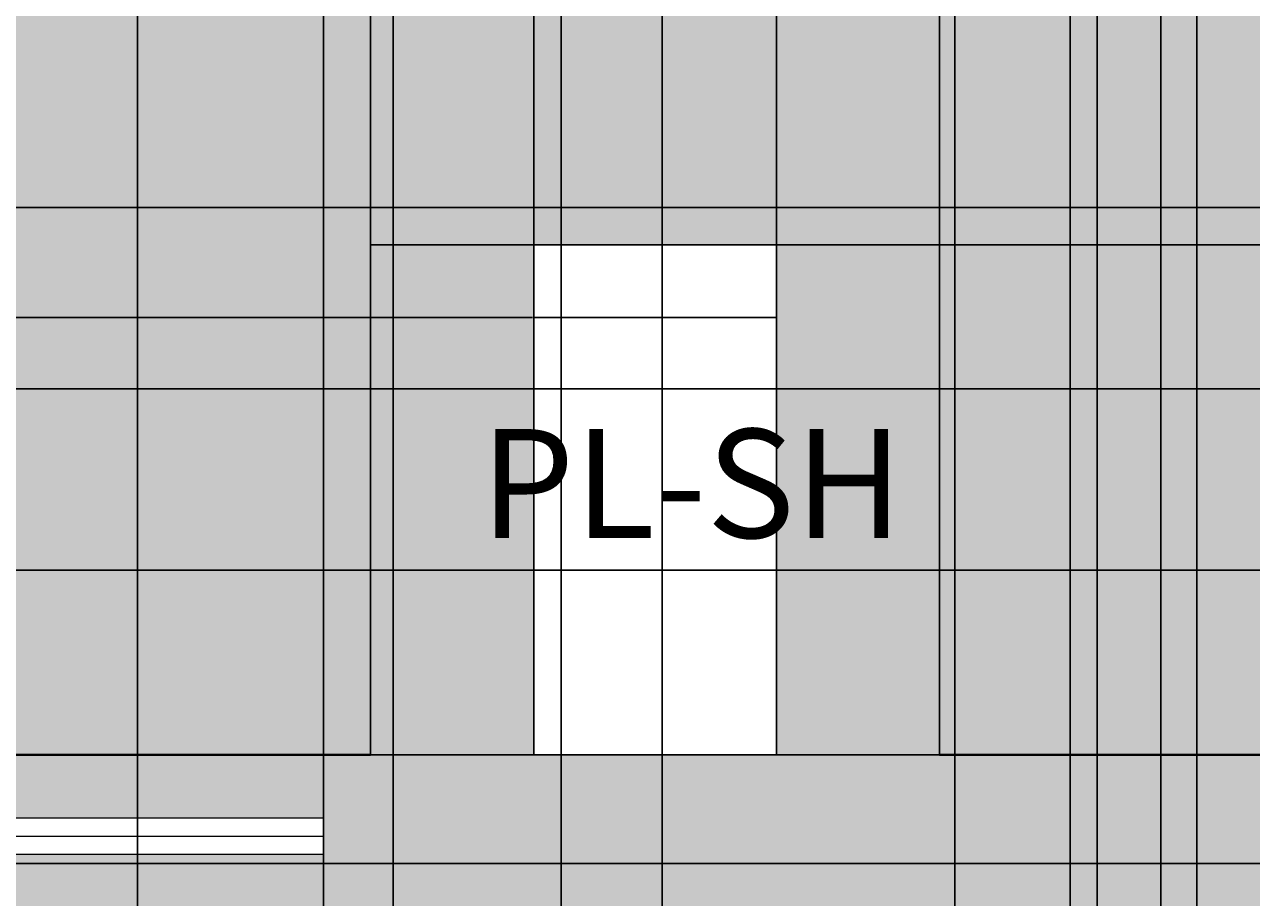
# Model space of a CAD drawing. Units: inches. Extents: x 818 to 1898, y 976 to 2364.
# Tile 77 of 96: x 1372 to 1439, y 2045 to 2093. Entities that reach past the tile are written whole.
import ezdxf

# ---------------------------------------------------------------- set-up
doc = ezdxf.new("R2010")
doc.units = ezdxf.units.IN
doc.header["$LTSCALE"] = 5
doc.header["$MEASUREMENT"] = 0
for name, color, linetype, lineweight in [('A-ANNO-DIMS', 2, 'Continuous', 18), ('A-ANNO-TEXT', 7, 'Continuous', 18), ('A-FLOR-SHFT', 7, 'Continuous', 25), ('A-GLAZ', 4, 'Continuous', 18), ('A-WALL', 7, 'Continuous', 40)]:
    doc.layers.add(name, color=color, linetype=linetype, lineweight=lineweight)
for name, color, linetype, lineweight, true_color in [('A-GLAZ-PATT', 141, 'Continuous', 9, 0xadddf7), ('A-WALL-PATT', 251, 'Continuous', 13, 0x636466), ('L-PLNT-PATT', 114, 'Continuous', 9, 0x139b48)]:
    doc.layers.add(name, color=color, linetype=linetype, lineweight=lineweight, true_color=true_color)
doc.styles.get("Standard").update_dxf_attribs({"font": 'arial.ttf'})
doc.dimstyles.get("Standard").update_dxf_attribs({"dimtxt": 0.18, "dimasz": 0.18, "dimexe": 0.18, "dimexo": 0.0625, "dimgap": 0.09, "dimtad": 0, "dimtih": 1, "dimtoh": 1, "dimdec": 4, "dimzin": 0, "dimdsep": 46, "dimtxsty": 'Standard', "dimcen": 0.09, "dimadec": 0, "dimazin": 0, "dimtfac": 1, "dimtdec": 4, "dimtofl": 0, "dimtmove": 0, "dimatfit": 3, "dimfxl": 1, "dimtolj": 1, "dimtzin": 0, "dimarcsym": 0})

# ---------------------------------------------------------------- blocks, each defined once
blk = doc.blocks.new('*D61')
at = {"layer": 'A-ANNO-DIMS', "color": 0, "lineweight": -2, "ltscale": 5, "transparency": 16777216}
for p, q in [((1071.725, 1203.027), (1071.725, 2363.873)), ((1071.905, 2363.693), (1250.936, 2363.693)), ((1430.545, 2363.693), (1251.514, 2363.693)), ((1430.725, 1203.027), (1430.725, 2363.873))]:
    blk.add_line(p, q, dxfattribs=at)
at = {"layer": 'A-ANNO-DIMS', "color": 0, "ltscale": 5, "transparency": 16777216}
for points in [[(1071.905, 2363.723), (1071.905, 2363.663), (1071.725, 2363.693)], [(1430.545, 2363.723), (1430.545, 2363.663), (1430.725, 2363.693)]]:
    blk.add_solid(points, dxfattribs=at)
at = {"layer": 'Defpoints', "color": 0, "ltscale": 5, "transparency": 16777216}
for p in [(1430.725, 2363.693), (1071.725, 1202.964), (1430.725, 1202.964)]:
    blk.add_point(p, dxfattribs=at)
at = {"layer": 'A-ANNO-DIMS', "color": 0, "ltscale": 5, "transparency": 16777216, "insert": (1251.225, 2363.693), "char_height": 0.18, "attachment_point": 5}
blk.add_mtext('\\A1;359', dxfattribs=at)
blk = doc.blocks.new('*D64')
at = {"layer": 'A-ANNO-DIMS', "color": 0, "lineweight": -2, "ltscale": 5, "transparency": 16777216}
for p, q in [((1197.725, 1501.141), (1197.725, 2363.873)), ((1197.905, 2363.693), (1313.935, 2363.693)), ((1430.545, 2363.693), (1314.516, 2363.693)), ((1430.725, 1501.141), (1430.725, 2363.873))]:
    blk.add_line(p, q, dxfattribs=at)
at = {"layer": 'A-ANNO-DIMS', "color": 0, "ltscale": 5, "transparency": 16777216}
for points in [[(1197.905, 2363.723), (1197.905, 2363.663), (1197.725, 2363.693)], [(1430.545, 2363.723), (1430.545, 2363.663), (1430.725, 2363.693)]]:
    blk.add_solid(points, dxfattribs=at)
at = {"layer": 'Defpoints', "color": 0, "ltscale": 5, "transparency": 16777216}
for p in [(1430.725, 2363.693), (1197.725, 1501.078), (1430.725, 1501.078)]:
    blk.add_point(p, dxfattribs=at)
at = {"layer": 'A-ANNO-DIMS', "color": 0, "ltscale": 5, "transparency": 16777216, "insert": (1314.225, 2363.693), "char_height": 0.18, "attachment_point": 5}
blk.add_mtext('\\A1;233', dxfattribs=at)
blk = doc.blocks.new('*D85')
at = {"layer": 'A-ANNO-DIMS', "color": 0, "lineweight": -2, "ltscale": 5, "transparency": 16777216}
for p, q in [((1258.788, 2053.078), (1897.916, 2053.078)), ((1897.736, 2052.898), (1897.736, 1876.76)), ((1897.736, 1700.258), (1897.736, 1876.396)), ((1258.788, 1700.078), (1897.916, 1700.078))]:
    blk.add_line(p, q, dxfattribs=at)
at = {"layer": 'A-ANNO-DIMS', "color": 0, "ltscale": 5, "transparency": 16777216}
for points in [[(1897.706, 2052.898), (1897.766, 2052.898), (1897.736, 2053.078)], [(1897.706, 1700.258), (1897.766, 1700.258), (1897.736, 1700.078)]]:
    blk.add_solid(points, dxfattribs=at)
at = {"layer": 'Defpoints', "color": 0, "ltscale": 5, "transparency": 16777216}
for p in [(1258.725, 2053.078), (1897.736, 2053.078), (1258.725, 1700.078)]:
    blk.add_point(p, dxfattribs=at)
at = {"layer": 'A-ANNO-DIMS', "color": 0, "ltscale": 5, "transparency": 16777216, "insert": (1897.736, 1876.578), "char_height": 0.18, "attachment_point": 5}
blk.add_mtext('\\A1;353', dxfattribs=at)
blk = doc.blocks.new('*D86')
at = {"layer": 'A-ANNO-DIMS', "color": 0, "lineweight": -2, "ltscale": 5, "transparency": 16777216}
for p, q in [((1258.725, 2053.141), (1258.725, 2363.873)), ((1258.905, 2363.693), (1486.433, 2363.693)), ((1714.545, 2363.693), (1487.018, 2363.693)), ((1714.725, 2053.141), (1714.725, 2363.873))]:
    blk.add_line(p, q, dxfattribs=at)
at = {"layer": 'A-ANNO-DIMS', "color": 0, "ltscale": 5, "transparency": 16777216}
for points in [[(1258.905, 2363.723), (1258.905, 2363.663), (1258.725, 2363.693)], [(1714.545, 2363.723), (1714.545, 2363.663), (1714.725, 2363.693)]]:
    blk.add_solid(points, dxfattribs=at)
at = {"layer": 'Defpoints', "color": 0, "ltscale": 5, "transparency": 16777216}
for p in [(1714.725, 2363.693), (1258.725, 2053.078), (1714.725, 2053.078)]:
    blk.add_point(p, dxfattribs=at)
at = {"layer": 'A-ANNO-DIMS', "color": 0, "ltscale": 5, "transparency": 16777216, "insert": (1486.725, 2363.693), "char_height": 0.18, "attachment_point": 5}
blk.add_mtext('\\A1;456', dxfattribs=at)
blk = doc.blocks.new('*D98')
at = {"layer": 'A-ANNO-DIMS', "color": 0, "lineweight": -2, "ltscale": 5, "transparency": 16777216}
for p, q in [((1338.541, 1071.118), (1338.541, 2363.873)), ((1338.721, 2363.693), (1364.815, 2363.693)), ((1391.696, 2363.693), (1365.602, 2363.693)), ((1391.876, 1071.118), (1391.876, 2363.873))]:
    blk.add_line(p, q, dxfattribs=at)
at = {"layer": 'A-ANNO-DIMS', "color": 0, "ltscale": 5, "transparency": 16777216}
for points in [[(1338.721, 2363.723), (1338.721, 2363.663), (1338.541, 2363.693)], [(1391.696, 2363.723), (1391.696, 2363.663), (1391.876, 2363.693)]]:
    blk.add_solid(points, dxfattribs=at)
at = {"layer": 'Defpoints', "color": 0, "ltscale": 5, "transparency": 16777216}
for p in [(1391.876, 2363.693), (1338.541, 1071.055), (1391.876, 1071.055)]:
    blk.add_point(p, dxfattribs=at)
at = {"layer": 'A-ANNO-DIMS', "color": 0, "ltscale": 5, "transparency": 16777216, "insert": (1365.208, 2363.693), "char_height": 0.18, "attachment_point": 5}
blk.add_mtext('\\A1;53.33', dxfattribs=at)
blk = doc.blocks.new('*D99')
at = {"layer": 'A-ANNO-DIMS', "color": 0, "lineweight": -2, "ltscale": 5, "transparency": 16777216}
for p, q in [((1391.876, 1071.118), (1391.876, 2363.873)), ((1392.056, 2363.693), (1420.454, 2363.693)), ((1449.64, 2363.693), (1421.241, 2363.693)), ((1449.82, 1071.118), (1449.82, 2363.873))]:
    blk.add_line(p, q, dxfattribs=at)
at = {"layer": 'A-ANNO-DIMS', "color": 0, "ltscale": 5, "transparency": 16777216}
for points in [[(1392.056, 2363.723), (1392.056, 2363.663), (1391.876, 2363.693)], [(1449.64, 2363.723), (1449.64, 2363.663), (1449.82, 2363.693)]]:
    blk.add_solid(points, dxfattribs=at)
at = {"layer": 'Defpoints', "color": 0, "ltscale": 5, "transparency": 16777216}
for p in [(1449.82, 2363.693), (1391.876, 1071.055), (1449.82, 1071.055)]:
    blk.add_point(p, dxfattribs=at)
at = {"layer": 'A-ANNO-DIMS', "color": 0, "ltscale": 5, "transparency": 16777216, "insert": (1420.848, 2363.693), "char_height": 0.18, "attachment_point": 5}
blk.add_mtext('\\A1;57.94', dxfattribs=at)
blk = doc.blocks.new('*D141')
at = {"layer": 'A-ANNO-DIMS', "color": 0, "lineweight": -2, "ltscale": 5, "transparency": 16777216}
for p, q in [((1218.174, 2083.262), (1897.916, 2083.262)), ((1897.736, 2083.082), (1897.736, 2073.444)), ((1897.736, 2063.442), (1897.736, 2073.08)), ((1198.174, 2063.262), (1897.916, 2063.262))]:
    blk.add_line(p, q, dxfattribs=at)
at = {"layer": 'A-ANNO-DIMS', "color": 0, "ltscale": 5, "transparency": 16777216}
for points in [[(1897.706, 2083.082), (1897.766, 2083.082), (1897.736, 2083.262)], [(1897.706, 2063.442), (1897.766, 2063.442), (1897.736, 2063.262)]]:
    blk.add_solid(points, dxfattribs=at)
at = {"layer": 'Defpoints', "color": 0, "ltscale": 5, "transparency": 16777216}
for p in [(1218.111, 2083.262), (1198.111, 2063.262), (1897.736, 2063.262)]:
    blk.add_point(p, dxfattribs=at)
at = {"layer": 'A-ANNO-DIMS', "color": 0, "ltscale": 5, "transparency": 16777216, "insert": (1897.736, 2073.262), "char_height": 0.18, "attachment_point": 5}
blk.add_mtext('\\A1;20', dxfattribs=at)
blk = doc.blocks.new('*D142')
at = {"layer": 'A-ANNO-DIMS', "color": 0, "lineweight": -2, "ltscale": 5, "transparency": 16777216}
for p, q in [((1208.174, 2073.262), (1897.916, 2073.262)), ((1897.736, 2073.082), (1897.736, 2068.444)), ((1897.736, 2063.442), (1897.736, 2068.08)), ((1198.174, 2063.262), (1897.916, 2063.262))]:
    blk.add_line(p, q, dxfattribs=at)
at = {"layer": 'A-ANNO-DIMS', "color": 0, "ltscale": 5, "transparency": 16777216}
for points in [[(1897.706, 2073.082), (1897.766, 2073.082), (1897.736, 2073.262)], [(1897.706, 2063.442), (1897.766, 2063.442), (1897.736, 2063.262)]]:
    blk.add_solid(points, dxfattribs=at)
at = {"layer": 'Defpoints', "color": 0, "ltscale": 5, "transparency": 16777216}
for p in [(1208.111, 2073.262), (1897.736, 2073.262), (1198.111, 2063.262)]:
    blk.add_point(p, dxfattribs=at)
at = {"layer": 'A-ANNO-DIMS', "color": 0, "ltscale": 5, "transparency": 16777216, "insert": (1897.736, 2068.262), "char_height": 0.18, "attachment_point": 5}
blk.add_mtext('\\A1;10', dxfattribs=at)
blk = doc.blocks.new('*D161')
at = {"layer": 'A-ANNO-DIMS', "color": 0, "lineweight": -2, "ltscale": 5, "transparency": 16777216}
for p, q in [((1429.225, 1876.141), (1429.225, 2363.873)), ((1429.405, 2363.693), (1509.589, 2363.693)), ((1590.545, 2363.693), (1510.361, 2363.693)), ((1590.725, 1876.141), (1590.725, 2363.873))]:
    blk.add_line(p, q, dxfattribs=at)
at = {"layer": 'A-ANNO-DIMS', "color": 0, "ltscale": 5, "transparency": 16777216}
for points in [[(1429.405, 2363.723), (1429.405, 2363.663), (1429.225, 2363.693)], [(1590.545, 2363.723), (1590.545, 2363.663), (1590.725, 2363.693)]]:
    blk.add_solid(points, dxfattribs=at)
at = {"layer": 'Defpoints', "color": 0, "ltscale": 5, "transparency": 16777216}
for p in [(1590.725, 2363.693), (1429.225, 1876.078), (1590.725, 1876.078)]:
    blk.add_point(p, dxfattribs=at)
at = {"layer": 'A-ANNO-DIMS', "color": 0, "ltscale": 5, "transparency": 16777216, "insert": (1509.975, 2363.693), "char_height": 0.18, "attachment_point": 5}
blk.add_mtext('\\A1;161.5', dxfattribs=at)
blk = doc.blocks.new('*D166')
at = {"layer": 'A-ANNO-DIMS', "color": 0, "lineweight": -2, "ltscale": 5, "transparency": 16777216}
for p, q in [((1401.146, 1510.141), (1401.146, 2363.873)), ((1401.326, 2363.693), (1415.54, 2363.693)), ((1430.545, 2363.693), (1416.331, 2363.693)), ((1430.725, 1510.141), (1430.725, 2363.873))]:
    blk.add_line(p, q, dxfattribs=at)
at = {"layer": 'A-ANNO-DIMS', "color": 0, "ltscale": 5, "transparency": 16777216}
for points in [[(1401.326, 2363.723), (1401.326, 2363.663), (1401.146, 2363.693)], [(1430.545, 2363.723), (1430.545, 2363.663), (1430.725, 2363.693)]]:
    blk.add_solid(points, dxfattribs=at)
at = {"layer": 'Defpoints', "color": 0, "ltscale": 5, "transparency": 16777216}
for p in [(1430.725, 2363.693), (1401.146, 1510.078), (1430.725, 1510.078)]:
    blk.add_point(p, dxfattribs=at)
at = {"layer": 'A-ANNO-DIMS', "color": 0, "ltscale": 5, "transparency": 16777216, "insert": (1415.936, 2363.693), "char_height": 0.18, "attachment_point": 5}
blk.add_mtext('\\A1;29.58', dxfattribs=at)
blk = doc.blocks.new('*D191')
at = {"layer": 'A-ANNO-DIMS', "color": 0, "lineweight": -2, "ltscale": 5, "transparency": 16777216}
for p, q in [((1434.225, 1409.115), (1434.225, 2363.873)), ((1434.405, 2363.693), (1435.076, 2363.693)), ((1436.045, 2363.693), (1435.375, 2363.693)), ((1436.225, 1409.115), (1436.225, 2363.873))]:
    blk.add_line(p, q, dxfattribs=at)
at = {"layer": 'A-ANNO-DIMS', "color": 0, "ltscale": 5, "transparency": 16777216}
for points in [[(1434.405, 2363.723), (1434.405, 2363.663), (1434.225, 2363.693)], [(1436.045, 2363.723), (1436.045, 2363.663), (1436.225, 2363.693)]]:
    blk.add_solid(points, dxfattribs=at)
at = {"layer": 'Defpoints', "color": 0, "ltscale": 5, "transparency": 16777216}
for p in [(1436.225, 2363.693), (1434.225, 1409.052), (1436.225, 1409.052)]:
    blk.add_point(p, dxfattribs=at)
at = {"layer": 'A-ANNO-DIMS', "color": 0, "ltscale": 5, "transparency": 16777216, "insert": (1435.225, 2363.693), "char_height": 0.18, "attachment_point": 5}
blk.add_mtext('\\A1;2', dxfattribs=at)
blk = doc.blocks.new('*D252')
at = {"layer": 'A-ANNO-DIMS', "color": 0, "lineweight": -2, "ltscale": 5, "transparency": 16777216}
for p, q in [((1330.305, 2053.016), (1330.305, 975.663)), ((1388.031, 2053.016), (1388.031, 975.663)), ((1330.485, 975.843), (1358.775, 975.843)), ((1387.851, 975.843), (1359.562, 975.843))]:
    blk.add_line(p, q, dxfattribs=at)
at = {"layer": 'A-ANNO-DIMS', "color": 0, "ltscale": 5, "transparency": 16777216}
for points in [[(1330.485, 975.873), (1330.485, 975.813), (1330.305, 975.843)], [(1387.851, 975.873), (1387.851, 975.813), (1388.031, 975.843)]]:
    blk.add_solid(points, dxfattribs=at)
at = {"layer": 'Defpoints', "color": 0, "ltscale": 5, "transparency": 16777216}
for p in [(1330.305, 2053.078), (1388.031, 2053.078), (1388.031, 975.843)]:
    blk.add_point(p, dxfattribs=at)
at = {"layer": 'A-ANNO-DIMS', "color": 0, "ltscale": 5, "transparency": 16777216, "insert": (1359.168, 975.843), "char_height": 0.18, "attachment_point": 5}
blk.add_mtext('\\A1;57.73', dxfattribs=at)
blk = doc.blocks.new('*D255')
at = {"layer": 'A-ANNO-DIMS', "color": 0, "lineweight": -2, "ltscale": 5, "transparency": 16777216}
for p, q in [((1388.031, 2053.141), (1388.031, 2363.873)), ((1388.211, 2363.693), (1388.939, 2363.693)), ((1390.456, 2363.693), (1389.728, 2363.693)), ((1390.636, 2053.141), (1390.636, 2363.873))]:
    blk.add_line(p, q, dxfattribs=at)
at = {"layer": 'A-ANNO-DIMS', "color": 0, "ltscale": 5, "transparency": 16777216}
for points in [[(1388.211, 2363.723), (1388.211, 2363.663), (1388.031, 2363.693)], [(1390.456, 2363.723), (1390.456, 2363.663), (1390.636, 2363.693)]]:
    blk.add_solid(points, dxfattribs=at)
at = {"layer": 'Defpoints', "color": 0, "ltscale": 5, "transparency": 16777216}
for p in [(1390.636, 2363.693), (1388.031, 2053.078), (1390.636, 2053.078)]:
    blk.add_point(p, dxfattribs=at)
at = {"layer": 'A-ANNO-DIMS', "color": 0, "ltscale": 5, "transparency": 16777216, "insert": (1389.334, 2363.693), "char_height": 0.18, "attachment_point": 5}
blk.add_mtext('\\A1;2.604', dxfattribs=at)
blk = doc.blocks.new('*D256')
at = {"layer": 'A-ANNO-DIMS', "color": 0, "lineweight": -2, "ltscale": 5, "transparency": 16777216}
for p, q in [((1399.636, 2053.141), (1399.636, 2363.873)), ((1399.816, 2363.693), (1405.873, 2363.693)), ((1412.84, 2363.693), (1406.783, 2363.693)), ((1413.02, 2077.251), (1413.02, 2363.873))]:
    blk.add_line(p, q, dxfattribs=at)
at = {"layer": 'A-ANNO-DIMS', "color": 0, "ltscale": 5, "transparency": 16777216}
for points in [[(1399.816, 2363.723), (1399.816, 2363.663), (1399.636, 2363.693)], [(1412.84, 2363.723), (1412.84, 2363.663), (1413.02, 2363.693)]]:
    blk.add_solid(points, dxfattribs=at)
at = {"layer": 'Defpoints', "color": 0, "ltscale": 5, "transparency": 16777216}
for p in [(1413.02, 2363.693), (1413.02, 2077.188), (1399.636, 2053.078)]:
    blk.add_point(p, dxfattribs=at)
at = {"layer": 'A-ANNO-DIMS', "color": 0, "ltscale": 5, "transparency": 16777216, "insert": (1406.328, 2363.693), "char_height": 0.18, "attachment_point": 5}
blk.add_mtext('\\A1;13.384', dxfattribs=at)
blk = doc.blocks.new('*D257')
at = {"layer": 'A-ANNO-DIMS', "color": 0, "lineweight": -2, "ltscale": 5, "transparency": 16777216}
for p, q in [((1399.573, 2077.188), (818.026, 2077.188)), ((818.206, 2077.008), (818.206, 2065.314)), ((818.206, 2053.258), (818.206, 2064.953)), ((1399.573, 2053.078), (818.026, 2053.078))]:
    blk.add_line(p, q, dxfattribs=at)
at = {"layer": 'A-ANNO-DIMS', "color": 0, "ltscale": 5, "transparency": 16777216}
for points in [[(818.176, 2077.008), (818.236, 2077.008), (818.206, 2077.188)], [(818.176, 2053.258), (818.236, 2053.258), (818.206, 2053.078)]]:
    blk.add_solid(points, dxfattribs=at)
at = {"layer": 'Defpoints', "color": 0, "ltscale": 5, "transparency": 16777216}
for p in [(818.206, 2077.188), (1399.636, 2077.188), (1399.636, 2053.078)]:
    blk.add_point(p, dxfattribs=at)
at = {"layer": 'A-ANNO-DIMS', "color": 0, "ltscale": 5, "transparency": 16777216, "insert": (818.206, 2065.133), "char_height": 0.18, "attachment_point": 5}
blk.add_mtext('\\A1;24.11', dxfattribs=at)
blk = doc.blocks.new('*D258')
at = {"layer": 'A-ANNO-DIMS', "color": 0, "lineweight": -2, "ltscale": 5, "transparency": 16777216}
for p, q in [((1422.02, 2053.141), (1422.02, 2363.873)), ((1422.2, 2363.693), (1453.264, 2363.693)), ((1484.942, 2363.693), (1453.878, 2363.693)), ((1485.122, 2053.141), (1485.122, 2363.873))]:
    blk.add_line(p, q, dxfattribs=at)
at = {"layer": 'A-ANNO-DIMS', "color": 0, "ltscale": 5, "transparency": 16777216}
for points in [[(1422.2, 2363.723), (1422.2, 2363.663), (1422.02, 2363.693)], [(1484.942, 2363.723), (1484.942, 2363.663), (1485.122, 2363.693)]]:
    blk.add_solid(points, dxfattribs=at)
at = {"layer": 'Defpoints', "color": 0, "ltscale": 5, "transparency": 16777216}
for p in [(1485.122, 2363.693), (1422.02, 2053.078), (1485.122, 2053.078)]:
    blk.add_point(p, dxfattribs=at)
at = {"layer": 'A-ANNO-DIMS', "color": 0, "ltscale": 5, "transparency": 16777216, "insert": (1453.571, 2363.693), "char_height": 0.18, "attachment_point": 5}
blk.add_mtext('\\A1;63.1', dxfattribs=at)
blk = doc.blocks.new('*D266')
at = {"layer": 'A-ANNO-DIMS', "color": 0, "lineweight": -2, "ltscale": 5, "transparency": 16777216}
for p, q in [((1780.439, 2053.078), (818.026, 2053.078)), ((818.206, 2052.898), (818.206, 2050.26)), ((818.206, 2047.258), (818.206, 2049.896)), ((1780.439, 2047.078), (818.026, 2047.078))]:
    blk.add_line(p, q, dxfattribs=at)
at = {"layer": 'A-ANNO-DIMS', "color": 0, "ltscale": 5, "transparency": 16777216}
for points in [[(818.176, 2052.898), (818.236, 2052.898), (818.206, 2053.078)], [(818.176, 2047.258), (818.236, 2047.258), (818.206, 2047.078)]]:
    blk.add_solid(points, dxfattribs=at)
at = {"layer": 'Defpoints', "color": 0, "ltscale": 5, "transparency": 16777216}
for p in [(1780.502, 2053.078), (818.206, 2047.078), (1780.502, 2047.078)]:
    blk.add_point(p, dxfattribs=at)
at = {"layer": 'A-ANNO-DIMS', "color": 0, "ltscale": 5, "transparency": 16777216, "insert": (818.206, 2050.078), "char_height": 0.18, "attachment_point": 5}
blk.add_mtext('\\A1;6', dxfattribs=at)
blk = doc.blocks.new('*D273')
at = {"layer": 'A-ANNO-DIMS', "color": 0, "lineweight": -2, "ltscale": 5, "transparency": 16777216}
for p, q in [((1406.725, 1587.479), (1406.725, 2363.873)), ((1406.905, 2363.693), (1418.505, 2363.693)), ((1430.545, 2363.693), (1418.945, 2363.693)), ((1430.725, 1587.479), (1430.725, 2363.873))]:
    blk.add_line(p, q, dxfattribs=at)
at = {"layer": 'A-ANNO-DIMS', "color": 0, "ltscale": 5, "transparency": 16777216}
for points in [[(1406.905, 2363.723), (1406.905, 2363.663), (1406.725, 2363.693)], [(1430.545, 2363.723), (1430.545, 2363.663), (1430.725, 2363.693)]]:
    blk.add_solid(points, dxfattribs=at)
at = {"layer": 'Defpoints', "color": 0, "ltscale": 5, "transparency": 16777216}
for p in [(1430.725, 2363.693), (1406.725, 1587.416), (1430.725, 1587.416)]:
    blk.add_point(p, dxfattribs=at)
at = {"layer": 'A-ANNO-DIMS', "color": 0, "ltscale": 5, "transparency": 16777216, "insert": (1418.725, 2363.693), "char_height": 0.18, "attachment_point": 5}
blk.add_mtext('\\A1;24', dxfattribs=at)
blk = doc.blocks.new('*D274')
at = {"layer": 'A-ANNO-DIMS', "color": 0, "lineweight": -2, "ltscale": 5, "transparency": 16777216}
for p, q in [((1311.025, 1897.929), (1311.025, 2363.873)), ((1311.205, 2363.693), (1344.007, 2363.693)), ((1377.599, 2363.693), (1344.797, 2363.693)), ((1377.779, 1897.929), (1377.779, 2363.873))]:
    blk.add_line(p, q, dxfattribs=at)
at = {"layer": 'A-ANNO-DIMS', "color": 0, "ltscale": 5, "transparency": 16777216}
for points in [[(1311.205, 2363.723), (1311.205, 2363.663), (1311.025, 2363.693)], [(1377.599, 2363.723), (1377.599, 2363.663), (1377.779, 2363.693)]]:
    blk.add_solid(points, dxfattribs=at)
at = {"layer": 'Defpoints', "color": 0, "ltscale": 5, "transparency": 16777216}
for p in [(1377.779, 2363.693), (1311.025, 1897.866), (1377.779, 1897.866)]:
    blk.add_point(p, dxfattribs=at)
at = {"layer": 'A-ANNO-DIMS', "color": 0, "ltscale": 5, "transparency": 16777216, "insert": (1344.402, 2363.693), "char_height": 0.18, "attachment_point": 5}
blk.add_mtext('\\A1;66.75', dxfattribs=at)
blk = doc.blocks.new('*D281')
at = {"layer": 'A-ANNO-DIMS', "color": 0, "lineweight": -2, "ltscale": 5, "transparency": 16777216}
for p, q in [((1250.303, 1913.703), (1250.303, 2363.873)), ((1250.483, 2363.693), (1420.121, 2363.693)), ((1590.545, 2363.693), (1420.907, 2363.693)), ((1590.725, 2011.141), (1590.725, 2363.873))]:
    blk.add_line(p, q, dxfattribs=at)
at = {"layer": 'A-ANNO-DIMS', "color": 0, "ltscale": 5, "transparency": 16777216}
for points in [[(1250.483, 2363.723), (1250.483, 2363.663), (1250.303, 2363.693)], [(1590.545, 2363.723), (1590.545, 2363.663), (1590.725, 2363.693)]]:
    blk.add_solid(points, dxfattribs=at)
at = {"layer": 'Defpoints', "color": 0, "ltscale": 5, "transparency": 16777216}
for p in [(1590.725, 2363.693), (1590.725, 2011.078), (1250.303, 1913.64)]:
    blk.add_point(p, dxfattribs=at)
at = {"layer": 'A-ANNO-DIMS', "color": 0, "ltscale": 5, "transparency": 16777216, "insert": (1420.514, 2363.693), "char_height": 0.18, "attachment_point": 5}
blk.add_mtext('\\A1;340.4', dxfattribs=at)
blk = doc.blocks.new('*D282')
at = {"layer": 'A-ANNO-DIMS', "color": 0, "lineweight": -2, "ltscale": 5, "transparency": 16777216}
for p, q in [((1422.083, 2081.188), (1897.916, 2081.188)), ((1897.736, 2081.008), (1897.736, 1884.315)), ((1897.736, 1687.258), (1897.736, 1883.951)), ((1463.788, 1687.078), (1897.916, 1687.078))]:
    blk.add_line(p, q, dxfattribs=at)
at = {"layer": 'A-ANNO-DIMS', "color": 0, "ltscale": 5, "transparency": 16777216}
for points in [[(1897.706, 2081.008), (1897.766, 2081.008), (1897.736, 2081.188)], [(1897.706, 1687.258), (1897.766, 1687.258), (1897.736, 1687.078)]]:
    blk.add_solid(points, dxfattribs=at)
at = {"layer": 'Defpoints', "color": 0, "ltscale": 5, "transparency": 16777216}
for p in [(1422.02, 2081.188), (1897.736, 2081.188), (1463.725, 1687.078)]:
    blk.add_point(p, dxfattribs=at)
at = {"layer": 'A-ANNO-DIMS', "color": 0, "ltscale": 5, "transparency": 16777216, "insert": (1897.736, 1884.133), "char_height": 0.18, "attachment_point": 5}
blk.add_mtext('\\A1;394.1', dxfattribs=at)
blk = doc.blocks.new('*D288')
at = {"layer": 'A-ANNO-DIMS', "color": 0, "lineweight": -2, "ltscale": 5, "transparency": 16777216}
for p, q in [((1422.876, 1742.674), (1422.876, 2363.873)), ((1423.056, 2363.693), (1466.906, 2363.693)), ((1511.545, 2363.693), (1467.695, 2363.693)), ((1511.725, 1716.108), (1511.725, 2363.873))]:
    blk.add_line(p, q, dxfattribs=at)
at = {"layer": 'A-ANNO-DIMS', "color": 0, "ltscale": 5, "transparency": 16777216}
for points in [[(1423.056, 2363.723), (1423.056, 2363.663), (1422.876, 2363.693)], [(1511.545, 2363.723), (1511.545, 2363.663), (1511.725, 2363.693)]]:
    blk.add_solid(points, dxfattribs=at)
at = {"layer": 'Defpoints', "color": 0, "ltscale": 5, "transparency": 16777216}
for p in [(1511.725, 2363.693), (1422.876, 1742.611), (1511.725, 1716.045)]:
    blk.add_point(p, dxfattribs=at)
at = {"layer": 'A-ANNO-DIMS', "color": 0, "ltscale": 5, "transparency": 16777216, "insert": (1467.3, 2363.693), "char_height": 0.18, "attachment_point": 5}
blk.add_mtext('\\A1;88.85', dxfattribs=at)

msp = doc.modelspace()

# ---------------------------------------------------------------- hatches: boundary and pattern name
at = {"layer": 'A-GLAZ-PATT', "ltscale": 5}
h = msp.add_hatch(color=256, dxfattribs=at)
h.dxf.hatch_style = 1
h.paths.add_polyline_path([(1283.8183, 1504.5782), (1206.7252, 1504.5782), (1206.7252, 1501.0782), (1283.8183, 1501.0782)])
h.paths.add_polyline_path([(1283.8183, 1510.0782), (1206.7252, 1510.0782), (1206.7252, 1506.5782), (1283.8183, 1506.5782)])
h.paths.add_polyline_path([(1490.9163, 1355.0782), (1439.7252, 1355.0782), (1439.7252, 1409.0522), (1436.2251, 1409.0522), (1436.2251, 1351.5782), (1490.9163, 1351.5782)])
h.paths.add_polyline_path([(1434.2251, 1409.0522), (1430.7251, 1409.0522), (1430.7251, 1346.0782), (1435.0799, 1346.0782), (1435.0731, 1346.1152), (1435.1501, 1346.0782), (1490.9163, 1346.0782), (1490.9163, 1349.5782), (1434.2251, 1349.5782)])
h.paths.add_polyline_path([(1714.7251, 1545.0782), (1711.2252, 1545.0782), (1711.2252, 1521.0782), (1714.7251, 1521.0782)])
h.paths.add_polyline_path([(1709.2252, 1545.0782), (1705.7252, 1545.0782), (1705.7252, 1521.0782), (1709.2252, 1521.0782)])
h.paths.add_polyline_path([(1714.7251, 1687.0782), (1711.2252, 1687.0782), (1711.2252, 1649.9029), (1714.7251, 1649.9029)])
h.paths.add_polyline_path([(1709.2252, 1687.0782), (1705.7252, 1687.0782), (1705.7252, 1649.9029), (1709.2252, 1649.9029)])
h.paths.add_polyline_path([(1709.2252, 1745.5584), (1705.7252, 1745.5584), (1705.7252, 1717.3178), (1709.2252, 1717.3178)])
h.paths.add_polyline_path([(1714.7251, 1745.5584), (1711.2252, 1745.5584), (1711.2252, 1717.3178), (1714.7251, 1717.3178)])
h.paths.add_polyline_path([(1714.7251, 2014.5114), (1711.2252, 2014.5114), (1711.2252, 1962.0338), (1714.7251, 1962.0338)])
h.paths.add_polyline_path([(1709.2252, 2014.5114), (1705.7252, 2014.5114), (1705.7252, 1962.0338), (1709.2252, 1962.0338)])
h.paths.add_polyline_path([(1538.5155, 2047.5782), (1485.1216, 2047.5782), (1485.1216, 2044.0782), (1538.5155, 2044.0782)])
h.paths.add_polyline_path([(1538.5155, 2053.0782), (1485.1216, 2053.0782), (1485.1216, 2049.5782), (1538.5155, 2049.5782)])
h.paths.add_polyline_path([(1388.0315, 2047.5782), (1330.305, 2047.5782), (1330.305, 2044.0782), (1388.0315, 2044.0782)])
h.paths.add_polyline_path([(1388.0315, 2053.0782), (1330.305, 2053.0782), (1330.305, 2049.5782), (1388.0315, 2049.5782)])
h.paths.add_polyline_path([(1262.2252, 2019.2871), (1258.7251, 2019.2871), (1258.7251, 1928.9218), (1262.2252, 1928.9218)])
h.paths.add_polyline_path([(1267.7252, 2019.2871), (1264.2252, 2019.2871), (1264.2252, 1928.9218), (1267.7252, 1928.9218)])
h.paths.add_polyline_path([(1262.2252, 1862.9652), (1258.7251, 1862.9652), (1258.7251, 1814.9652), (1262.2252, 1814.9652)])
h.paths.add_polyline_path([(1267.7252, 1862.9652), (1264.2252, 1862.9652), (1264.2252, 1814.9652), (1267.7252, 1814.9652)])
h.paths.add_polyline_path([(1262.2252, 1755.3321), (1258.7251, 1755.3321), (1258.7251, 1707.3321), (1262.2252, 1707.3321)])
h.paths.add_polyline_path([(1267.7252, 1755.3321), (1264.2252, 1755.3321), (1264.2252, 1707.3321), (1267.7252, 1707.3321)])
h.paths.add_polyline_path([(1251.9333, 1692.5782), (1206.7252, 1692.5782), (1206.7252, 1687.0782), (1251.9333, 1687.0782)])
h.paths.add_polyline_path([(1251.9333, 1700.0782), (1206.7252, 1700.0782), (1206.7252, 1694.5782), (1251.9333, 1694.5782)])
at = {"layer": 'A-WALL-PATT', "ltscale": 5}
h = msp.add_hatch(color=256, dxfattribs=at)
h.dxf.hatch_style = 1
h.paths.add_polyline_path([(1267.7252, 1928.9218), (1258.7251, 1928.9218), (1258.7251, 1913.6401), (1250.3029, 1913.6401), (1250.3029, 1878.3919), (1258.7251, 1878.3919), (1258.7251, 1862.9652), (1267.7252, 1862.9652)])
h.paths.add_polyline_path([(1267.7252, 1814.9652), (1258.7251, 1814.9652), (1258.7251, 1755.3321), (1267.7252, 1755.3321)])
h.paths.add_polyline_path([(1463.7251, 1696.0782), (1267.7252, 1696.0782), (1267.7252, 1707.3321), (1258.7251, 1707.3321), (1258.7251, 1700.0782), (1251.9333, 1700.0782), (1251.9333, 1687.0782), (1463.7251, 1687.0782)])
h.paths.add_polyline_path([(1714.7251, 1717.3178), (1705.7252, 1717.3178), (1705.7252, 1696.0782), (1599.7252, 1696.0782), (1599.7252, 1790.0782), (1705.7252, 1790.0782), (1705.7252, 1785.6125), (1714.7251, 1785.6125), (1714.7251, 1827.2125), (1705.7252, 1827.2125), (1705.7252, 1802.0782), (1599.7252, 1802.0782), (1599.7252, 1867.0782), (1705.7252, 1867.0782), (1705.7252, 1857.2125), (1714.7251, 1857.2125), (1714.7251, 1930.0316), (1741.8409, 1930.0316), (1741.8409, 1935.0316), (1714.7251, 1935.0316), (1714.7251, 1957.0338), (1741.8409, 1957.0338), (1741.8409, 1962.0338), (1714.7251, 1962.0338), (1705.7252, 1962.0338), (1705.7252, 1948.0782), (1599.7252, 1948.0782), (1599.7252, 1981.0782), (1590.7251, 1981.0782), (1590.7251, 1941.0782), (1620.7252, 1941.0782), (1705.7252, 1941.0782), (1705.7252, 1876.0782), (1599.7252, 1876.0782), (1599.7252, 1911.0782), (1590.7251, 1911.0782), (1590.7251, 1876.0782), (1429.2251, 1876.0782), (1429.2251, 1867.0782), (1511.7251, 1867.0782), (1528.593, 1867.0782), (1595.7252, 1867.0782), (1595.7252, 1773.0782), (1520.7252, 1773.0782), (1520.7252, 1837.5823), (1532.593, 1837.5823), (1532.593, 1867.0782), (1528.593, 1867.0782), (1528.593, 1841.5823), (1511.7251, 1841.5823), (1511.7251, 1744.9714), (1520.7252, 1744.9714), (1520.7252, 1761.0782), (1595.7252, 1761.0782), (1595.7252, 1696.0782), (1520.7252, 1696.0782), (1520.7252, 1716.0454), (1511.7251, 1716.0454), (1511.7251, 1696.0782), (1511.7251, 1687.0782), (1714.7251, 1687.0782)])
h.paths.add_polyline_path([(1714.7251, 2053.0782), (1714.7251, 2081.1881), (1709.7252, 2081.1881), (1709.7252, 2053.0782), (1681.6446, 2053.0782), (1681.6446, 2081.1881), (1676.6446, 2081.1881), (1676.6446, 2053.0782), (1538.5155, 2053.0782), (1538.5155, 2044.0782), (1590.7251, 2044.0782), (1590.7251, 2011.0782), (1599.7252, 2011.0782), (1599.7252, 2044.0782), (1705.7252, 2044.0782), (1705.7252, 2014.5114), (1714.7251, 2014.5114)])
h.paths.add_polyline_path([(1485.1216, 2053.0782), (1422.02, 2053.0782), (1422.02, 2081.1881), (1413.02, 2081.1881), (1413.02, 2053.0782), (1399.6356, 2053.0782), (1399.6356, 2081.1881), (1390.6356, 2081.1881), (1390.6356, 2053.0782), (1388.0315, 2053.0782), (1388.0315, 2044.0782), (1416.2743, 2044.0782), (1485.1216, 2044.0782)])
h.paths.add_polyline_path([(1330.305, 2053.0782), (1258.7251, 2053.0782), (1258.7251, 2019.2871), (1267.7252, 2019.2871), (1267.7252, 2044.0782), (1330.305, 2044.0782)])
h.paths.add_polyline_path([(1258.7251, 2053.0782), (1214.6577, 2053.0782), (1214.6577, 2044.0782), (1258.7251, 2044.0782)])
h.paths.add_polyline_path([(1214.6577, 2053.0782), (1180.349, 2053.0782), (1180.349, 2044.0782), (1214.6577, 2044.0782)])
h.paths.add_polyline_path([(1714.7251, 1639.5782), (1741.8409, 1639.5782), (1741.8409, 1643.5782), (1714.7251, 1643.5782), (1714.7251, 1649.9029), (1705.7252, 1649.9029), (1705.7252, 1600.0782), (1477.7252, 1600.0782), (1477.7252, 1591.0782), (1520.7252, 1591.0782), (1616.7252, 1591.0782), (1616.7252, 1416.6857), (1622.7252, 1416.6857), (1622.7252, 1463.0782), (1624.7252, 1463.0782), (1624.7252, 1467.0782), (1622.7252, 1467.0782), (1622.7252, 1591.0782), (1705.7252, 1591.0782), (1705.7252, 1545.0782), (1714.7251, 1545.0782), (1741.8409, 1545.0782), (1741.8409, 1549.0782), (1714.7251, 1549.0782), (1714.7251, 1593.9175), (1737.8409, 1593.9175), (1737.8409, 1597.9175), (1714.7251, 1597.9175)])
h.paths.add_polyline_path([(1674.9024, 2060.7419), (1714.7045, 2060.7419), (1714.7045, 2073.1061), (1674.9024, 2073.1061)], flags=25)
h.paths.add_polyline_path([(1394.5468, 2061.6618), (1422.2344, 2061.6618), (1422.2344, 2074.0261), (1394.5468, 2074.0261)], flags=24)
at = {"layer": 'L-PLNT-PATT', "ltscale": 5}
h = msp.add_hatch(color=256, dxfattribs=at)
h.dxf.hatch_style = 1
h.paths.add_polyline_path([(1789.7173, 2205.9709), (1083.7252, 2205.9709), (1083.7252, 2083.2623), (1218.1114, 2083.2623), (1218.1114, 2053.0782), (1390.6356, 2053.0782), (1390.6356, 2081.1881), (1399.6356, 2081.1881), (1413.02, 2081.1881), (1422.02, 2081.1881), (1422.02, 2053.0782), (1676.6446, 2053.0782), (1676.6446, 2081.1881), (1714.7251, 2081.1881), (1714.7251, 2081.6235), (1789.7173, 2081.6235)])
h.paths.add_polyline_path([(1388.6037, 2145.2461), (1388.6037, 2122.3767), (1373.4756, 2122.3767), (1373.4756, 2145.2461)], flags=16)
h.paths.add_polyline_path([(1408.6922, 2145.2461), (1423.8203, 2145.2461), (1423.8203, 2122.3767), (1408.6922, 2122.3767)], flags=16)
h.paths.add_polyline_path([(1353.3871, 2155.7839), (1353.3871, 2122.3767), (1338.259, 2122.3767), (1338.259, 2155.7839)], flags=16)
h.paths.add_polyline_path([(1443.9089, 2158.4222), (1459.037, 2158.4222), (1459.037, 2122.3767), (1443.9089, 2122.3767)], flags=16)
h.paths.add_polyline_path([(1318.1705, 2145.2461), (1318.1705, 2122.3767), (1303.0424, 2122.3767), (1303.0424, 2145.2461)], flags=16)
h.paths.add_polyline_path([(1479.1255, 2145.2461), (1494.2536, 2145.2461), (1494.2536, 2122.3767), (1479.1255, 2122.3767)], flags=16)
h.paths.add_polyline_path([(1282.9539, 2145.2461), (1282.9539, 2122.3767), (1267.8258, 2122.3767), (1267.8258, 2145.2461)], flags=16)
h.paths.add_polyline_path([(1514.3421, 2145.2461), (1529.4702, 2145.2461), (1529.4702, 2122.3767), (1514.3421, 2122.3767)], flags=16)
h.paths.add_polyline_path([(1247.7373, 2159.4296), (1247.7373, 2122.3767), (1232.6091, 2122.3767), (1232.6091, 2159.4296)], flags=16)
h.paths.add_polyline_path([(1549.5587, 2156.9246), (1564.6868, 2156.9246), (1564.6868, 2122.3767), (1549.5587, 2122.3767)], flags=16)
h.paths.add_polyline_path([(1212.5206, 2145.2461), (1212.5206, 2122.3767), (1197.3925, 2122.3767), (1197.3925, 2145.2461)], flags=16)
h.paths.add_polyline_path([(1584.7753, 2145.2461), (1599.9034, 2145.2461), (1599.9034, 2122.3767), (1584.7753, 2122.3767)], flags=16)
h.paths.add_polyline_path([(1185.1073, 2104.7786), (1190.6407, 2104.7786), (1185.1073, 2098.2505), (1179.5738, 2104.7786)], flags=16)
h.paths.add_polyline_path([(1619.9919, 2145.2461), (1635.1201, 2145.2461), (1635.1201, 2122.3767), (1619.9919, 2122.3767)], flags=16)
h.paths.add_polyline_path([(1655.2086, 2156.1761), (1670.3367, 2156.1761), (1670.3367, 2122.3767), (1655.2086, 2122.3767)], flags=16)
h.paths.add_polyline_path([(1686.5992, 2145.2461), (1701.7273, 2145.2461), (1701.7273, 2122.3767), (1686.5992, 2122.3767)], flags=16)
h.paths.add_polyline_path([(1715.7616, 2145.2461), (1730.8897, 2145.2461), (1730.8897, 2122.3767), (1715.7616, 2122.3767)], flags=16)
h.paths.add_polyline_path([(1753.1652, 2145.2461), (1776.3312, 2145.2461), (1776.3312, 2115.6891), (1753.1652, 2115.6891)], flags=16)
h.paths.add_polyline_path([(1191.4331, 2146.5159), (1176.7891, 2146.5159), (1176.7891, 2134.1516), (1191.4331, 2134.1516)], flags=24)

# ---------------------------------------------------------------- linework, layer by layer
at = {"layer": 'A-FLOR-SHFT'}
for p, q in [((1390.6356, 2053.0782), (1390.6356, 2081.1881)), ((1390.6356, 2081.1881), (1399.6356, 2081.1881)), ((1399.6356, 2053.0782), (1399.6356, 2081.1881)), ((1399.6356, 2081.1881), (1413.02, 2081.1881)), ((1413.02, 2053.0782), (1413.02, 2081.1881)), ((1413.02, 2081.1881), (1422.02, 2081.1881)), ((1422.02, 2053.0782), (1422.02, 2081.1881)), ((1399.6356, 2077.1881), (1413.02, 2077.1881)), ((1399.6356, 2053.0782), (1413.02, 2053.0782))]:
    msp.add_line(p, q, dxfattribs=at)
at = {"layer": 'A-GLAZ'}
for p, q in [((1388.0315, 2053.0782), (1388.0315, 2044.0782)), ((1388.0315, 2049.5782), (1330.305, 2049.5782)), ((1388.0315, 2048.5782), (1330.305, 2048.5782)), ((1388.0315, 2047.5782), (1330.305, 2047.5782))]:
    msp.add_line(p, q, dxfattribs=at)
at = {"layer": 'A-WALL'}
for p, q in [((1083.7252, 2053.0782), (1390.6356, 2053.0782)), ((1422.02, 2053.0782), (1676.6446, 2053.0782))]:
    msp.add_line(p, q, dxfattribs=at)

# ---------------------------------------------------------------- texts
at = {"layer": 'A-ANNO-TEXT', "ltscale": 5, "insert": (1396.6935, 2071.0404), "char_height": 6, "attachment_point": 1}
msp.add_mtext_dynamic_manual_height_columns('PL-SH', width=118.992422, gutter_width=1, heights=[0], dxfattribs=at)

# ---------------------------------------------------------------- dimensions: what is measured, and where the dimension line sits
at = {"layer": 'A-ANNO-DIMS', "ltscale": 5}
for base, p1, p2, override, picture, middle in [((1430.7251, 2363.6929), (1071.7251, 1202.9642), (1430.7251, 1202.9642), {"dimdec": 0, "dimlfac": 1, "dimrnd": 0, "dimzin": 0, "dimdsep": 46, "dimlunit": 2}, '*D61', (1251.2251, 2363.6929)), ((1430.7251, 2363.6929), (1197.7251, 1501.0782), (1430.7251, 1501.0782), {"dimdec": 0, "dimlfac": 1, "dimrnd": 0, "dimzin": 0, "dimdsep": 46, "dimlunit": 2}, '*D64', (1314.2251, 2363.6929)), ((1590.7251, 2363.6929), (1250.3029, 1913.6401), (1590.7251, 2011.0782), {"dimdec": 1, "dimlfac": 1, "dimrnd": 0, "dimzin": 0, "dimdsep": 46, "dimlunit": 2}, '*D281', (1420.514, 2363.6929)), ((1714.7251, 2363.6929), (1258.7251, 2053.0782), (1714.7251, 2053.0782), {"dimdec": 0, "dimlfac": 1, "dimrnd": 0, "dimzin": 0, "dimdsep": 46, "dimlunit": 2}, '*D86', (1486.7251, 2363.6929)), ((1377.7791, 2363.6929), (1311.025, 1897.8663), (1377.7791, 1897.8663), {"dimdec": 2, "dimlfac": 1, "dimrnd": 0, "dimzin": 0, "dimdsep": 46, "dimlunit": 2}, '*D274', (1344.4021, 2363.6929)), ((1391.8757, 2363.6929), (1338.5412, 1071.0552), (1391.8757, 1071.0552), {"dimdec": 2, "dimlfac": 1, "dimrnd": 0, "dimzin": 0, "dimdsep": 46, "dimlunit": 2}, '*D98', (1365.2084, 2363.6929)), ((1390.6356, 2363.6929), (1388.0315, 2053.0782), (1390.6356, 2053.0782), {"dimdec": 3, "dimlfac": 1, "dimrnd": 0, "dimzin": 0, "dimdsep": 46, "dimlunit": 2}, '*D255', (1389.3335, 2363.6929)), ((1449.8196, 2363.6929), (1391.8757, 1071.0552), (1449.8196, 1071.0552), {"dimdec": 2, "dimlfac": 1, "dimrnd": 0, "dimzin": 0, "dimdsep": 46, "dimlunit": 2}, '*D99', (1420.8477, 2363.6929)), ((1413.02, 2363.6929), (1399.6356, 2053.0782), (1413.02, 2077.1881), {"dimdec": 3, "dimlfac": 1, "dimrnd": 0, "dimzin": 0, "dimdsep": 46, "dimlunit": 2}, '*D256', (1406.3278, 2363.6929)), ((1430.7251, 2363.6929), (1401.1463, 1510.0782), (1430.7251, 1510.0782), {"dimdec": 2, "dimlfac": 1, "dimrnd": 0, "dimzin": 0, "dimdsep": 46, "dimlunit": 2}, '*D166', (1415.9357, 2363.6929)), ((1430.7251, 2363.6929), (1406.7251, 1587.4164), (1430.7251, 1587.4164), {"dimdec": 0, "dimlfac": 1, "dimrnd": 0, "dimzin": 0, "dimdsep": 46, "dimlunit": 2}, '*D273', (1418.7251, 2363.6929)), ((1485.1216, 2363.6929), (1422.02, 2053.0782), (1485.1216, 2053.0782), {"dimdec": 1, "dimlfac": 1, "dimrnd": 0, "dimzin": 0, "dimdsep": 46, "dimlunit": 2}, '*D258', (1453.5708, 2363.6929)), ((1511.7251, 2363.6929), (1422.8756, 1742.6113), (1511.7251, 1716.0454), {"dimdec": 2, "dimlfac": 1, "dimrnd": 0, "dimzin": 0, "dimdsep": 46, "dimlunit": 2}, '*D288', (1467.3004, 2363.6929)), ((1590.7251, 2363.6929), (1429.2251, 1876.0782), (1590.7251, 1876.0782), {"dimdec": 1, "dimlfac": 1, "dimrnd": 0, "dimzin": 0, "dimdsep": 46, "dimlunit": 2}, '*D161', (1509.9751, 2363.6929)), ((1436.2251, 2363.6929), (1434.2251, 1409.0522), (1436.2251, 1409.0522), {"dimdec": 0, "dimlfac": 1, "dimrnd": 0, "dimzin": 0, "dimdsep": 46, "dimlunit": 2}, '*D191', (1435.2251, 2363.6929)), ((1388.0315, 975.8433), (1330.305, 2053.0782), (1388.0315, 2053.0782), {"dimdec": 2, "dimlfac": 1, "dimrnd": 0, "dimzin": 0, "dimdsep": 46, "dimlunit": 2}, '*D252', (1359.1682, 975.8433))]:
    dim = msp.add_linear_dim(base=base, p1=p1, p2=p2, dimstyle='Standard', override=override, dxfattribs=at)
    dim.commit()
    dim.dimension.update_dxf_attribs({"geometry": picture, "text_midpoint": middle})
for base, p1, p2, override, picture, middle in [((1897.736, 2063.2623), (1218.1114, 2083.2623), (1198.1114, 2063.2623), {"dimdec": 0, "dimlfac": 1, "dimrnd": 0, "dimzin": 0, "dimdsep": 46, "dimlunit": 2}, '*D141', (1897.736, 2073.2623)), ((1897.736, 2081.1881), (1463.7251, 1687.0782), (1422.02, 2081.1881), {"dimdec": 1, "dimlfac": 1, "dimrnd": 0, "dimzin": 0, "dimdsep": 46, "dimlunit": 2}, '*D282', (1897.736, 1884.1332)), ((818.2059, 2077.1881), (1399.6356, 2053.0782), (1399.6356, 2077.1881), {"dimdec": 2, "dimlfac": 1, "dimrnd": 0, "dimzin": 0, "dimdsep": 46, "dimlunit": 2}, '*D257', (818.2059, 2065.1332)), ((1897.736, 2073.2623), (1198.1114, 2063.2623), (1208.1114, 2073.2623), {"dimdec": 0, "dimlfac": 1, "dimrnd": 0, "dimzin": 0, "dimdsep": 46, "dimlunit": 2}, '*D142', (1897.736, 2068.2623)), ((818.2059, 2047.0782), (1780.5019, 2053.0782), (1780.5019, 2047.0782), {"dimdec": 0, "dimlfac": 1, "dimrnd": 0, "dimzin": 0, "dimdsep": 46, "dimlunit": 2}, '*D266', (818.2059, 2050.0782)), ((1897.736, 2053.0782), (1258.7251, 1700.0782), (1258.7251, 2053.0782), {"dimdec": 0, "dimlfac": 1, "dimrnd": 0, "dimzin": 0, "dimdsep": 46, "dimlunit": 2}, '*D85', (1897.736, 1876.5782))]:
    dim = msp.add_linear_dim(base=base, p1=p1, p2=p2, angle=90, dimstyle='Standard', override=override, dxfattribs=at)
    dim.commit()
    dim.dimension.update_dxf_attribs({"geometry": picture, "text_midpoint": middle})

doc.saveas('drawing.dxf')
